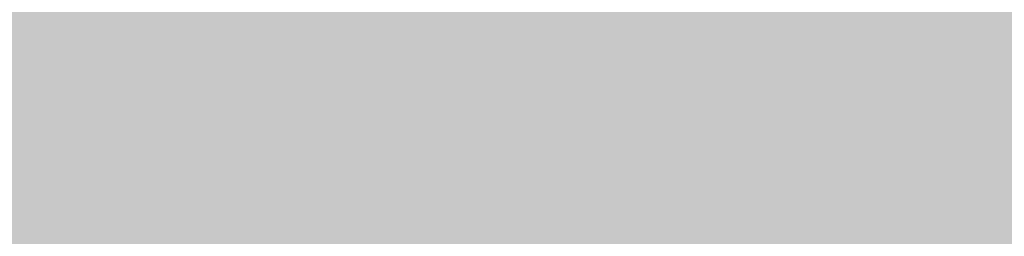
# Model space of a CAD drawing. Units: feet. Extents: x 3168 to 4724, y 827 to 1477.
# Tile 111 of 256: x 3284.48 to 3298.68, y 1093.65 to 1096.78. Entities that reach past the tile are written whole.
import ezdxf

# ---------------------------------------------------------------- set-up
doc = ezdxf.new("R2010")
doc.units = ezdxf.units.FT
doc.layers.add('A-ELEV-PATT', color=8, linetype='Continuous', lineweight=13)

msp = doc.modelspace()

# ---------------------------------------------------------------- hatches: boundary and pattern name
at = {"layer": 'A-ELEV-PATT'}
h = msp.add_hatch(color=256, dxfattribs=at)
h.dxf.hatch_style = 1
edge = h.paths.add_edge_path()
edge.add_ellipse((3552.906, 979.22), major_axis=(36.745, 0), ratio=0.484848, start_angle=0, end_angle=360)
edge = h.paths.add_edge_path()
edge.add_ellipse((3559.892, 929.252), major_axis=(36.745, 0), ratio=0.484848, start_angle=0, end_angle=360)
edge = h.paths.add_edge_path()
edge.add_line((3299.317, 1198.606), (3479.917, 1198.606))
edge.add_line((3479.917, 1198.606), (3479.917, 1209.869))
edge.add_spline(control_points=[(3479.917, 1209.869), (3464.301, 1209.869), (3448.686, 1209.869), (3410.949, 1209.869), (3388.828, 1209.869), (3355.647, 1209.869), (3344.586, 1209.869), (3327.996, 1209.869), (3322.466, 1209.869), (3314.17, 1209.869), (3311.405, 1209.869), (3307.257, 1209.869), (3305.875, 1209.869), (3303.801, 1209.869), (3303.11, 1209.869), (3302.073, 1209.869), (3301.727, 1209.869), (3301.209, 1209.869), (3301.036, 1209.869), (3300.777, 1209.869), (3300.69, 1209.869), (3300.561, 1209.869), (3300.517, 1209.869), (3300.453, 1209.869), (3300.431, 1209.869), (3300.399, 1209.869), (3300.388, 1209.869), (3300.366, 1209.869), (3300.346, 1209.869), (3300.346, 1209.869), (3300.346, 1209.869), (3300.343, 1209.869), (3300.341, 1209.869), (3300.338, 1209.869), (3300.337, 1209.869), (3300.334, 1209.869), (3300.332, 1209.869), (3300.326, 1209.869), (3300.321, 1209.869), (3300.311, 1209.869), (3300.306, 1209.869), (3300.291, 1209.869), (3300.28, 1209.869), (3300.232, 1209.869), (3300.195, 1209.869), (3299.951, 1209.871), (3299.745, 1209.874), (3299.437, 1209.883), (3299.334, 1209.887), (3299.181, 1209.893), (3299.13, 1209.895), (3298.652, 1209.917), (3298.229, 1209.946), (3297.602, 1210.002), (3297.393, 1210.023), (3297.083, 1210.058), (3296.979, 1210.07), (3296.293, 1210.155), (3295.718, 1210.243), (3294.869, 1210.399), (3294.588, 1210.454), (3294.169, 1210.543), (3294.03, 1210.574), (3291.707, 1211.101), (3289.654, 1211.813), (3285.776, 1213.564), (3283.951, 1214.603), (3280.512, 1216.98), (3278.897, 1218.318), (3276.38, 1220.829), (3275.416, 1221.918), (3274.039, 1223.708), (3273.581, 1224.35), (3273.143, 1225.016)], knot_values=[39.119033, 39.119033, 39.119033, 39.119033, 39.286353, 39.286353, 39.523379, 39.523379, 39.641892, 39.641892, 39.701148, 39.701148, 39.730777, 39.730777, 39.745591, 39.745591, 39.752998, 39.752998, 39.756701, 39.756701, 39.758553, 39.758553, 39.759479, 39.759479, 39.759942, 39.759942, 39.760173, 39.760173, 39.760289, 39.760289, 39.760405, 39.760405, 39.760463, 39.760463, 39.763389, 39.763389, 39.764851, 39.764851, 39.767304, 39.767304, 39.773825, 39.773825, 39.78057, 39.78057, 39.79477, 39.79477, 39.845194, 39.845194, 40.126715, 40.126715, 40.267476, 40.267476, 40.337856, 40.337856, 40.927023, 40.927023, 41.221606, 41.221606, 41.368898, 41.368898, 42.202622, 42.202622, 42.619485, 42.619485, 42.827916, 42.827916, 46.118323, 46.118323, 49.408731, 49.408731, 52.699139, 52.699139, 54.927489, 54.927489, 56.104228, 56.104228, 56.104228, 56.104228], weights=[1, 1, 1, 1, 1, 1, 1, 1, 1, 1, 1, 1, 1, 1, 1, 1, 1, 1, 1, 1, 1, 1, 1, 1, 1, 1, 1, 1, 1, 1, 1, 1, 1, 1, 1, 1, 1, 1, 1, 1, 1, 1, 1, 1, 1, 1, 1, 1, 1, 1, 1, 1, 1, 1, 1, 1, 1, 1, 1, 1, 1, 1, 1, 1, 1, 1, 1, 1, 1, 1, 1, 1, 1, 1], degree=3, periodic=0)
edge.add_line((3273.143, 1225.016), (3273.143, 1099.016))
edge.add_line((3273.143, 1099.016), (3299.317, 1099.016))
edge.add_line((3299.317, 1099.016), (3299.317, 1198.606))
edge = h.paths.add_edge_path()
edge.add_line((3304.758, 1324.158), (3479.917, 1324.158))
edge.add_line((3479.917, 1324.158), (3479.917, 1335.715))
edge.add_line((3479.917, 1335.715), (3269.162, 1335.715))
edge.add_spline(control_points=[(3269.162, 1335.715), (3264.024, 1335.715), (3258.364, 1328.958), (3259.264, 1323.9)], knot_values=[0, 0, 0, 0, 15.412191, 15.412191, 15.412191, 15.412191], degree=3, periodic=0)
edge.add_line((3259.264, 1323.9), (3265.517, 1288.769))
edge.add_line((3265.517, 1288.769), (3275.265, 1261.546))
edge.add_line((3275.265, 1261.546), (3304.758, 1261.546))
edge.add_line((3304.758, 1261.546), (3304.758, 1324.158))
h = msp.add_hatch(color=256, dxfattribs=at)
h.dxf.hatch_style = 1
h.paths.add_polyline_path([(3384.525, 1099.016), (3335.029, 1099.016), (3299.317, 1099.016), (3273.143, 1099.016), (3217.565, 1099.016), (3168.069, 827.116), (3335.029, 827.116)])

doc.saveas('drawing.dxf')
